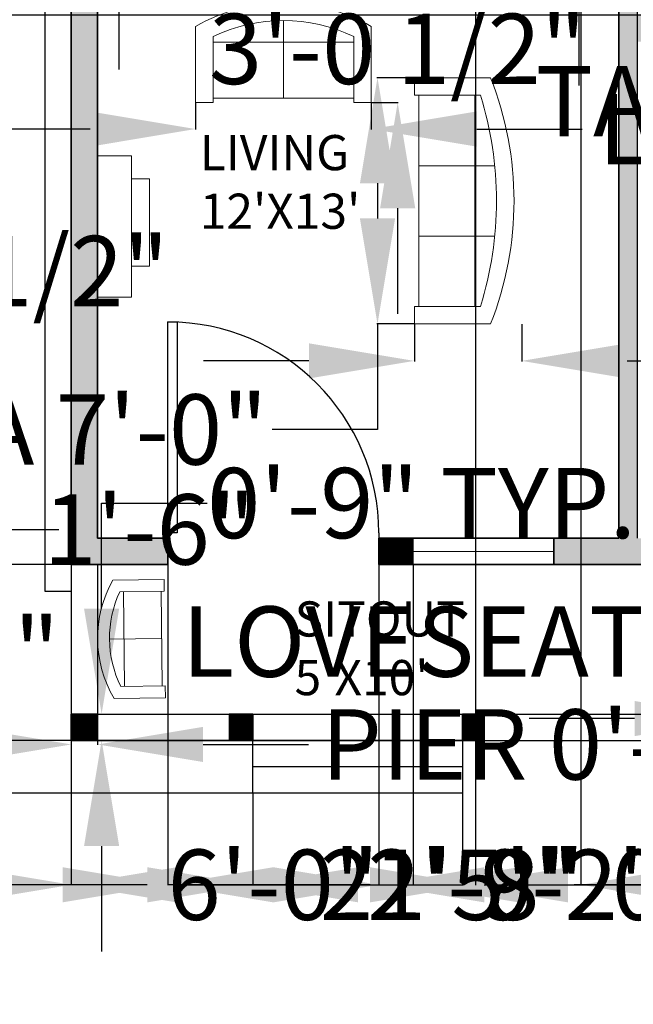
# Model space of a CAD drawing. Units: inches. Extents: x 2838 to 4029, y 1041 to 1915.
# Tile 2 of 16: x 3250 to 3460, y 1041 to 1377. Entities that reach past the tile are written whole.
import ezdxf

# ---------------------------------------------------------------- set-up
doc = ezdxf.new("R2010")
doc.units = ezdxf.units.IN
doc.header["$MEASUREMENT"] = 0
for name, color, linetype, lineweight in [('A-ANNO-DIMS', 2, 'Continuous', 18), ('A-AREA-IDEN', 7, 'Continuous', 18), ('A-COLS', 7, 'Continuous', 35), ('A-DOOR', 3, 'Continuous', 25), ('A-FLOR', 7, 'Continuous', 25), ('A-FLOR-STRS', 7, 'Continuous', 25), ('A-FURN', 8, 'Continuous', 18), ('A-GLAZ', 4, 'Continuous', 18), ('A-WALL', 7, 'Continuous', 35), ('A-WALL-PATT', 252, 'Continuous', 13)]:
    doc.layers.add(name, color=color, linetype=linetype, lineweight=lineweight)
doc.styles.get("Standard").update_dxf_attribs({"font": 'arial.ttf'})
doc.dimstyles.get("Standard").update_dxf_attribs({"dimtxt": 24, "dimasz": 36, "dimexe": 0.18, "dimexo": 0.0625, "dimgap": 0.09, "dimtad": 0, "dimtih": 1, "dimtoh": 1, "dimdec": 0, "dimzin": 0, "dimdsep": 46, "dimlunit": 3, "dimtxsty": 'Standard', "dimcen": 0.09, "dimadec": 0, "dimazin": 0, "dimtfac": 1, "dimtdec": 0, "dimtofl": 0, "dimtmove": 0, "dimatfit": 3, "dimfxl": 1, "dimtolj": 1, "dimtzin": 0, "dimarcsym": 0})

# ---------------------------------------------------------------- blocks, each defined once
blk = doc.blocks.new('*U4')
for p, q in [((0, 0), (0, -6)), ((40, 0), (40, -6))]:
    blk.add_line(p, q)
blk.add_lwpolyline([(0, 0), (0, 40), (1.75, 40), (1.75, 0)], close=True)
blk.add_arc((0, 0), 40, 0, 90)
blk = doc.blocks.new('Sofa - Roundback Loveseat 5 ft.')
for p, q in [((0, -32.44198), (0, -5.99998)), ((-24, -33.99998), (-24, -11.46958)), ((-23.9998, -13.38178), (23.99986, -13.38178)), ((24.00004, -33.99998), (24.00004, -11.46958)), ((-24, -32.44198), (24.00004, -32.44198))]:
    blk.add_line(p, q)
for points in [[(-24, -33.99998), (-30, -33.99998), (-30, -7.99998)], [(30.00004, -7.99998), (30.00004, -33.99998), (24.00004, -33.99998)]]:
    blk.add_lwpolyline(points)
for centre, radius, start, end in [((0, -60.24998), 60.24998, 60.13715, 119.8628), ((0, -61.38438), 55.38444, 64.32083, 115.6792)]:
    blk.add_arc(centre, radius, start, end)
blk = doc.blocks.new('Sofa - Roundback 7 ft.')
for p, q in [((-12.00002, -32.4421), (-12.00003, -6.5971)), ((11.99997, -32.4421), (11.99998, -6.5971)), ((-36.000027, -34), (-36.000027, -11.4696)), ((-35.999844, -13.3819), (35.9998, -13.3819)), ((35.99998, -34), (35.99998, -11.4696)), ((-36.000027, -32.4421), (35.99998, -32.4421))]:
    blk.add_line(p, q)
for points in [[(-36.000027, -34), (-42.000027, -34), (-42.000027, -8)], [(41.99998, -8), (41.99998, -34), (35.99998, -34)]]:
    blk.add_lwpolyline(points)
for centre, radius, start, end in [((0, -114.25), 114.25, 68.43141, 111.5686), ((-0.00001, -127.1968), 121.1968, 72.72033, 107.2797)]:
    blk.add_arc(centre, radius, start, end)
blk = doc.blocks.new('WIN-48')
blk.add_line((4.5, 48), (4.5, 0))
blk.add_lwpolyline([(0, 48), (9, 48), (9, 0), (0, 0)], close=True)
blk = doc.blocks.new('PORCH-PIER-9X9')
blk.add_lwpolyline([(9, 9), (0, 9), (0, 0), (9, 0)], close=True)
blk = doc.blocks.new('*D25')
at = {"layer": 'A-ANNO-DIMS', "color": 0, "lineweight": -2, "transparency": 16777216}
for p, q in [((3283.93, 1516.17), (3283.93, 1552.17)), ((3276.79, 1480.17), (3284.11, 1480.17)), ((3276.79, 1432.17), (3284.11, 1432.17)), ((3283.93, 1396.17), (3283.93, 1360.17))]:
    blk.add_line(p, q, dxfattribs=at)
at = {"layer": 'A-ANNO-DIMS', "color": 0, "transparency": 16777216}
for points in [[(3277.93, 1516.17), (3289.93, 1516.17), (3283.93, 1480.17)], [(3277.93, 1396.17), (3289.93, 1396.17), (3283.93, 1432.17)]]:
    blk.add_solid(points, dxfattribs=at)
at = {"layer": 'Defpoints', "color": 0, "transparency": 16777216}
for p in [(3276.73, 1480.17), (3283.93, 1480.17), (3276.73, 1432.17)]:
    blk.add_point(p, dxfattribs=at)
at = {"layer": 'A-ANNO-DIMS', "color": 0, "transparency": 16777216, "insert": (3283.93, 1456.17), "char_height": 24, "attachment_point": 5}
blk.add_mtext('\\A1;WINDOW 4\'-0" TYP.', dxfattribs=at)
blk = doc.blocks.new('*D29')
at = {"layer": 'A-ANNO-DIMS', "color": 0, "lineweight": -2, "transparency": 16777216}
for p, q in [((3310.15, 1348.85), (3310.15, 1339.73)), ((3370.15, 1348.85), (3370.15, 1339.73)), ((3274.15, 1339.91), (3238.15, 1339.91)), ((3406.15, 1339.91), (3442.15, 1339.91))]:
    blk.add_line(p, q, dxfattribs=at)
at = {"layer": 'A-ANNO-DIMS', "color": 0, "transparency": 16777216}
for points in [[(3274.15, 1345.91), (3274.15, 1333.91), (3310.15, 1339.91)], [(3406.15, 1345.91), (3406.15, 1333.91), (3370.15, 1339.91)]]:
    blk.add_solid(points, dxfattribs=at)
at = {"layer": 'Defpoints', "color": 0, "transparency": 16777216}
for p in [(3310.15, 1348.91), (3370.15, 1348.91), (3370.15, 1339.91)]:
    blk.add_point(p, dxfattribs=at)
at = {"layer": 'A-ANNO-DIMS', "color": 0, "transparency": 16777216, "insert": (3566.77, 1339.91), "char_height": 24, "attachment_point": 5}
blk.add_mtext('\\A1;LOVESEAT 5\'-0"', dxfattribs=at)
blk = doc.blocks.new('*D30')
at = {"layer": 'A-ANNO-DIMS', "color": 0, "lineweight": -2, "transparency": 16777216}
for p, q in [((3379.15, 1421.58), (3379.15, 1457.58)), ((3370.21, 1385.58), (3379.33, 1385.58)), ((3370.21, 1348.91), (3379.33, 1348.91)), ((3379.15, 1312.91), (3379.15, 1276.91))]:
    blk.add_line(p, q, dxfattribs=at)
at = {"layer": 'A-ANNO-DIMS', "color": 0, "transparency": 16777216}
for points in [[(3373.15, 1421.58), (3385.15, 1421.58), (3379.15, 1385.58)], [(3373.15, 1312.91), (3385.15, 1312.91), (3379.15, 1348.91)]]:
    blk.add_solid(points, dxfattribs=at)
at = {"layer": 'Defpoints', "color": 0, "transparency": 16777216}
for p in [(3370.15, 1385.58), (3379.15, 1385.58), (3370.15, 1348.91)]:
    blk.add_point(p, dxfattribs=at)
at = {"layer": 'A-ANNO-DIMS', "color": 0, "transparency": 16777216, "insert": (3379.15, 1367.25), "char_height": 24, "attachment_point": 5}
blk.add_mtext('\\A1;3\'-0 1/2"', dxfattribs=at)
blk = doc.blocks.new('*D31')
at = {"layer": 'A-ANNO-DIMS', "color": 0, "lineweight": -2, "transparency": 16777216}
for p, q in [((3489.98, 1221.23), (3489.98, 1257.23)), ((3495.97, 1185.23), (3489.8, 1185.23)), ((3495.97, 1144.84), (3489.8, 1144.84)), ((3489.98, 1108.84), (3489.98, 1072.84))]:
    blk.add_line(p, q, dxfattribs=at)
at = {"layer": 'A-ANNO-DIMS', "color": 0, "transparency": 16777216}
for points in [[(3483.98, 1221.23), (3495.98, 1221.23), (3489.98, 1185.23)], [(3483.98, 1108.84), (3495.98, 1108.84), (3489.98, 1144.84)]]:
    blk.add_solid(points, dxfattribs=at)
at = {"layer": 'Defpoints', "color": 0, "transparency": 16777216}
for p in [(3496.03, 1185.23), (3489.98, 1144.84), (3496.03, 1144.84)]:
    blk.add_point(p, dxfattribs=at)
at = {"layer": 'A-ANNO-DIMS', "color": 0, "transparency": 16777216, "insert": (3489.98, 1165.04), "char_height": 24, "attachment_point": 5}
blk.add_mtext('\\A1;LOVESEAT 3\'-4 1/2" TYP.', dxfattribs=at)
blk = doc.blocks.new('*D32')
at = {"layer": 'A-ANNO-DIMS', "color": 0, "lineweight": -2, "transparency": 16777216}
for p, q in [((3496.03, 1144.78), (3496.03, 1138.61)), ((3520.71, 1144.78), (3520.71, 1138.61)), ((3460.03, 1138.79), (3424.03, 1138.79)), ((3556.71, 1138.79), (3592.71, 1138.79))]:
    blk.add_line(p, q, dxfattribs=at)
at = {"layer": 'A-ANNO-DIMS', "color": 0, "transparency": 16777216}
for points in [[(3460.03, 1144.79), (3460.03, 1132.79), (3496.03, 1138.79)], [(3556.71, 1144.79), (3556.71, 1132.79), (3520.71, 1138.79)]]:
    blk.add_solid(points, dxfattribs=at)
at = {"layer": 'Defpoints', "color": 0, "transparency": 16777216}
for p in [(3496.03, 1144.84), (3520.71, 1144.84), (3520.71, 1138.79)]:
    blk.add_point(p, dxfattribs=at)
at = {"layer": 'A-ANNO-DIMS', "color": 0, "transparency": 16777216, "insert": (3694.12, 1138.79), "char_height": 24, "attachment_point": 5}
blk.add_mtext('\\A1;2\'-0 1/2" TYP.', dxfattribs=at)
blk = doc.blocks.new('*D33')
at = {"layer": 'A-ANNO-DIMS', "color": 0, "lineweight": -2, "transparency": 16777216}
for p, q in [((3601.73, 1469.45), (3601.73, 1505.45)), ((3603.48, 1433.45), (3601.55, 1433.45)), ((3603.48, 1421.37), (3601.55, 1421.37)), ((3601.73, 1385.37), (3601.73, 1349.37)), ((3601.73, 1349.37), (3565.73, 1349.37))]:
    blk.add_line(p, q, dxfattribs=at)
at = {"layer": 'A-ANNO-DIMS', "color": 0, "transparency": 16777216}
for points in [[(3595.73, 1469.45), (3607.73, 1469.45), (3601.73, 1433.45)], [(3595.73, 1385.37), (3607.73, 1385.37), (3601.73, 1421.37)]]:
    blk.add_solid(points, dxfattribs=at)
at = {"layer": 'Defpoints', "color": 0, "transparency": 16777216}
for p in [(3603.54, 1433.45), (3601.73, 1421.37), (3603.54, 1421.37)]:
    blk.add_point(p, dxfattribs=at)
at = {"layer": 'A-ANNO-DIMS', "color": 0, "transparency": 16777216, "insert": (3496.18, 1349.37), "char_height": 24, "attachment_point": 5}
blk.add_mtext('\\A1;TAP 1\'-0"', dxfattribs=at)
blk = doc.blocks.new('*D43')
at = {"layer": 'A-ANNO-DIMS', "color": 0, "lineweight": -2, "transparency": 16777216}
for p, q in [((3231.73, 1129.95), (3195.73, 1129.95)), ((3267.73, 1131.23), (3267.73, 1129.77)), ((3276.73, 1131.23), (3276.73, 1129.77)), ((3312.73, 1129.95), (3348.73, 1129.95))]:
    blk.add_line(p, q, dxfattribs=at)
at = {"layer": 'A-ANNO-DIMS', "color": 0, "transparency": 16777216}
for points in [[(3231.73, 1135.95), (3231.73, 1123.95), (3267.73, 1129.95)], [(3312.73, 1135.95), (3312.73, 1123.95), (3276.73, 1129.95)]]:
    blk.add_solid(points, dxfattribs=at)
at = {"layer": 'Defpoints', "color": 0, "transparency": 16777216}
for p in [(3267.73, 1131.3), (3276.73, 1131.3), (3276.73, 1129.95)]:
    blk.add_point(p, dxfattribs=at)
at = {"layer": 'A-ANNO-DIMS', "color": 0, "transparency": 16777216, "insert": (3465.15, 1129.95), "char_height": 24, "attachment_point": 5}
blk.add_mtext('\\A1;PIER 0\'-9" TYP.', dxfattribs=at)
blk = doc.blocks.new('*D44')
at = {"layer": 'A-ANNO-DIMS', "color": 0, "lineweight": -2, "transparency": 16777216}
for p, q in [((3278.08, 1176.3), (3278.08, 1212.3)), ((3278.08, 1212.3), (3314.08, 1212.3)), ((3276.79, 1140.3), (3278.26, 1140.3)), ((3276.79, 1131.3), (3278.26, 1131.3)), ((3278.08, 1095.3), (3278.08, 1059.3))]:
    blk.add_line(p, q, dxfattribs=at)
at = {"layer": 'A-ANNO-DIMS', "color": 0, "transparency": 16777216}
for points in [[(3272.08, 1176.3), (3284.08, 1176.3), (3278.08, 1140.3)], [(3272.08, 1095.3), (3284.08, 1095.3), (3278.08, 1131.3)]]:
    blk.add_solid(points, dxfattribs=at)
at = {"layer": 'Defpoints', "color": 0, "transparency": 16777216}
for p in [(3276.73, 1140.3), (3278.08, 1140.3), (3276.73, 1131.3)]:
    blk.add_point(p, dxfattribs=at)
at = {"layer": 'A-ANNO-DIMS', "color": 0, "transparency": 16777216, "insert": (3387.32, 1212.3), "char_height": 24, "attachment_point": 5}
blk.add_mtext('\\A1;0\'-9" TYP.', dxfattribs=at)
blk = doc.blocks.new('*D49')
at = {"layer": 'A-ANNO-DIMS', "color": 0, "lineweight": -2, "transparency": 16777216}
for p, q in [((3336.37, 1426.68), (3336.37, 1412.92)), ((3427.37, 1426.68), (3427.37, 1412.92)), ((3372.37, 1413.1), (3391.37, 1413.1)), ((3427.37, 1413.1), (3463.37, 1413.1))]:
    blk.add_line(p, q, dxfattribs=at)
at = {"layer": 'A-ANNO-DIMS', "color": 0, "transparency": 16777216}
for points in [[(3372.37, 1419.1), (3372.37, 1407.1), (3336.37, 1413.1)], [(3391.37, 1419.1), (3391.37, 1407.1), (3427.37, 1413.1)]]:
    blk.add_solid(points, dxfattribs=at)
at = {"layer": 'Defpoints', "color": 0, "transparency": 16777216}
for p in [(3336.37, 1426.75), (3427.37, 1426.75), (3427.37, 1413.1)]:
    blk.add_point(p, dxfattribs=at)
at = {"layer": 'A-ANNO-DIMS', "color": 0, "transparency": 16777216, "insert": (3595.36, 1413.1), "char_height": 24, "attachment_point": 5}
blk.add_mtext('\\A1;DINING SET 7\'-7"', dxfattribs=at)
blk = doc.blocks.new('*D50')
at = {"layer": 'A-ANNO-DIMS', "color": 0, "lineweight": -2, "transparency": 16777216}
for p, q in [((3441.02, 1517.75), (3441.02, 1553.75)), ((3427.44, 1481.75), (3441.2, 1481.75)), ((3427.44, 1426.75), (3441.2, 1426.75)), ((3441.02, 1390.75), (3441.02, 1354.75))]:
    blk.add_line(p, q, dxfattribs=at)
at = {"layer": 'A-ANNO-DIMS', "color": 0, "transparency": 16777216}
for points in [[(3435.02, 1517.75), (3447.02, 1517.75), (3441.02, 1481.75)], [(3435.02, 1390.75), (3447.02, 1390.75), (3441.02, 1426.75)]]:
    blk.add_solid(points, dxfattribs=at)
at = {"layer": 'Defpoints', "color": 0, "transparency": 16777216}
for p in [(3427.37, 1481.75), (3441.02, 1481.75), (3427.37, 1426.75)]:
    blk.add_point(p, dxfattribs=at)
at = {"layer": 'A-ANNO-DIMS', "color": 0, "transparency": 16777216, "insert": (3441.02, 1454.25), "char_height": 24, "attachment_point": 5}
blk.add_mtext('\\A1;4\'-7"', dxfattribs=at)
blk = doc.blocks.new('*D51')
at = {"layer": 'A-ANNO-DIMS', "color": 0, "lineweight": -2, "transparency": 16777216}
for p, q in [((3384.81, 1357.41), (3372.09, 1357.41)), ((3372.27, 1321.41), (3372.27, 1309.41)), ((3384.81, 1273.41), (3372.09, 1273.41)), ((3372.27, 1273.41), (3372.27, 1237.41)), ((3372.27, 1237.41), (3336.27, 1237.41))]:
    blk.add_line(p, q, dxfattribs=at)
at = {"layer": 'A-ANNO-DIMS', "color": 0, "transparency": 16777216}
for points in [[(3366.27, 1321.41), (3378.27, 1321.41), (3372.27, 1357.41)], [(3366.27, 1309.41), (3378.27, 1309.41), (3372.27, 1273.41)]]:
    blk.add_solid(points, dxfattribs=at)
at = {"layer": 'Defpoints', "color": 0, "transparency": 16777216}
for p in [(3384.87, 1357.41), (3372.27, 1273.41), (3384.87, 1273.41)]:
    blk.add_point(p, dxfattribs=at)
at = {"layer": 'A-ANNO-DIMS', "color": 0, "transparency": 16777216, "insert": (3254.04, 1237.41), "char_height": 24, "attachment_point": 5}
blk.add_mtext('\\A1;SOFA 7\'-0"', dxfattribs=at)
blk = doc.blocks.new('*D52')
at = {"layer": 'A-ANNO-DIMS', "color": 0, "lineweight": -2, "transparency": 16777216}
for p, q in [((3384.87, 1273.35), (3384.87, 1260.63)), ((3421.54, 1273.35), (3421.54, 1260.63)), ((3348.87, 1260.81), (3312.87, 1260.81)), ((3457.54, 1260.81), (3493.54, 1260.81))]:
    blk.add_line(p, q, dxfattribs=at)
at = {"layer": 'A-ANNO-DIMS', "color": 0, "transparency": 16777216}
for points in [[(3348.87, 1266.81), (3348.87, 1254.81), (3384.87, 1260.81)], [(3457.54, 1266.81), (3457.54, 1254.81), (3421.54, 1260.81)]]:
    blk.add_solid(points, dxfattribs=at)
at = {"layer": 'Defpoints', "color": 0, "transparency": 16777216}
for p in [(3384.87, 1273.41), (3421.54, 1273.41), (3421.54, 1260.81)]:
    blk.add_point(p, dxfattribs=at)
at = {"layer": 'A-ANNO-DIMS', "color": 0, "transparency": 16777216, "insert": (3553.48, 1260.81), "char_height": 24, "attachment_point": 5}
blk.add_mtext('\\A1;3\'-0 1/2"', dxfattribs=at)
blk = doc.blocks.new('*D57')
at = {"layer": 'A-ANNO-DIMS', "color": 0, "lineweight": -2, "transparency": 16777216}
for p, q in [((3585.57, 1472.38), (3585.57, 1508.38)), ((3590.9, 1436.38), (3585.39, 1436.38)), ((3590.9, 1400.38), (3585.39, 1400.38)), ((3585.57, 1364.38), (3585.57, 1328.38))]:
    blk.add_line(p, q, dxfattribs=at)
at = {"layer": 'A-ANNO-DIMS', "color": 0, "transparency": 16777216}
for points in [[(3579.57, 1472.38), (3591.57, 1472.38), (3585.57, 1436.38)], [(3579.57, 1364.38), (3591.57, 1364.38), (3585.57, 1400.38)]]:
    blk.add_solid(points, dxfattribs=at)
at = {"layer": 'Defpoints', "color": 0, "transparency": 16777216}
for p in [(3590.97, 1436.38), (3585.57, 1400.38), (3590.97, 1400.38)]:
    blk.add_point(p, dxfattribs=at)
at = {"layer": 'A-ANNO-DIMS', "color": 0, "transparency": 16777216, "insert": (3585.57, 1418.38), "char_height": 24, "attachment_point": 5}
blk.add_mtext('\\A1;DOUBLE SINK 3\'-0"', dxfattribs=at)
blk = doc.blocks.new('*D65')
at = {"layer": 'A-ANNO-DIMS', "color": 0, "lineweight": -2, "transparency": 16777216}
for p, q in [((3267.73, 1131.23), (3267.73, 1081.89)), ((3527.95, 1131.23), (3527.95, 1081.89)), ((3303.73, 1082.07), (3356.32, 1082.07)), ((3491.95, 1082.07), (3439.36, 1082.07))]:
    blk.add_line(p, q, dxfattribs=at)
at = {"layer": 'A-ANNO-DIMS', "color": 0, "transparency": 16777216}
for points in [[(3303.73, 1088.07), (3303.73, 1076.07), (3267.73, 1082.07)], [(3491.95, 1088.07), (3491.95, 1076.07), (3527.95, 1082.07)]]:
    blk.add_solid(points, dxfattribs=at)
at = {"layer": 'Defpoints', "color": 0, "transparency": 16777216}
for p in [(3267.73, 1131.3), (3527.95, 1131.3), (3527.95, 1082.07)]:
    blk.add_point(p, dxfattribs=at)
at = {"layer": 'A-ANNO-DIMS', "color": 0, "transparency": 16777216, "insert": (3397.84, 1082.07), "char_height": 24, "attachment_point": 5}
blk.add_mtext('\\A1;21\'-8"', dxfattribs=at)
blk = doc.blocks.new('*D66')
at = {"layer": 'A-ANNO-DIMS', "color": 0, "lineweight": -2, "transparency": 16777216}
for p, q in [((3227.506626, 1227.297346), (3227.506626, 1263.297346)), ((3267.669126, 1191.297346), (3227.326626, 1191.297346)), ((3267.669126, 1131.297346), (3227.326626, 1131.297346)), ((3227.506626, 1095.297346), (3227.506626, 1059.297346))]:
    blk.add_line(p, q, dxfattribs=at)
at = {"layer": 'A-ANNO-DIMS', "color": 0, "transparency": 16777216}
for points in [[(3221.506626, 1227.297346), (3233.506626, 1227.297346), (3227.506626, 1191.297346)], [(3221.506626, 1095.297346), (3233.506626, 1095.297346), (3227.506626, 1131.297346)]]:
    blk.add_solid(points, dxfattribs=at)
at = {"layer": 'Defpoints', "color": 0, "transparency": 16777216}
for p in [(3267.731626, 1191.297346), (3227.506626, 1131.297346), (3267.731626, 1131.297346)]:
    blk.add_point(p, dxfattribs=at)
at = {"layer": 'A-ANNO-DIMS', "color": 0, "transparency": 16777216, "insert": (3227.506626, 1161.297346), "char_height": 24, "attachment_point": 5}
blk.add_mtext('\\A1;5\'-0"', dxfattribs=at)
blk = doc.blocks.new('*D67')
at = {"layer": 'A-ANNO-DIMS', "color": 0, "lineweight": -2, "transparency": 16777216}
for p, q in [((3258.67, 1680.3), (3227.33, 1680.3)), ((3227.51, 1644.3), (3227.51, 1409.15)), ((3227.51, 1149.3), (3227.51, 1384.45)), ((3329.6, 1113.3), (3227.33, 1113.3))]:
    blk.add_line(p, q, dxfattribs=at)
at = {"layer": 'A-ANNO-DIMS', "color": 0, "transparency": 16777216}
for points in [[(3221.51, 1644.3), (3233.51, 1644.3), (3227.51, 1680.3)], [(3221.51, 1149.3), (3233.51, 1149.3), (3227.51, 1113.3)]]:
    blk.add_solid(points, dxfattribs=at)
at = {"layer": 'Defpoints', "color": 0, "transparency": 16777216}
for p in [(3227.51, 1680.3), (3258.73, 1680.3), (3329.66, 1113.3)]:
    blk.add_point(p, dxfattribs=at)
at = {"layer": 'A-ANNO-DIMS', "color": 0, "transparency": 16777216, "insert": (3227.51, 1396.8), "char_height": 24, "attachment_point": 5}
blk.add_mtext('\\A1;47\'-3"', dxfattribs=at)
blk = doc.blocks.new('*D69')
at = {"layer": 'A-ANNO-DIMS', "color": 0, "lineweight": -2, "transparency": 16777216}
for p, q in [((3300.731626, 1191.234846), (3300.731626, 1081.892346)), ((3372.731626, 1191.234846), (3372.731626, 1081.892346)), ((3264.731626, 1082.072346), (3228.731626, 1082.072346)), ((3408.731626, 1082.072346), (3444.731626, 1082.072346))]:
    blk.add_line(p, q, dxfattribs=at)
at = {"layer": 'A-ANNO-DIMS', "color": 0, "transparency": 16777216}
for points in [[(3264.731626, 1088.072346), (3264.731626, 1076.072346), (3300.731626, 1082.072346)], [(3408.731626, 1088.072346), (3408.731626, 1076.072346), (3372.731626, 1082.072346)]]:
    blk.add_solid(points, dxfattribs=at)
at = {"layer": 'Defpoints', "color": 0, "transparency": 16777216}
for p in [(3300.731626, 1191.297346), (3372.731626, 1191.297346), (3372.731626, 1082.072346)]:
    blk.add_point(p, dxfattribs=at)
at = {"layer": 'A-ANNO-DIMS', "color": 0, "transparency": 16777216, "insert": (3336.731626, 1082.072346), "char_height": 24, "attachment_point": 5}
blk.add_mtext('\\A1;6\'-0"', dxfattribs=at)
blk = doc.blocks.new('*D70')
at = {"layer": 'A-ANNO-DIMS', "color": 0, "lineweight": -2, "transparency": 16777216}
for p, q in [((3329.66, 1113.23), (3329.66, 1081.89)), ((3401.28, 1113.23), (3401.28, 1081.89)), ((3293.66, 1082.07), (3257.66, 1082.07)), ((3437.28, 1082.07), (3473.28, 1082.07))]:
    blk.add_line(p, q, dxfattribs=at)
at = {"layer": 'A-ANNO-DIMS', "color": 0, "transparency": 16777216}
for points in [[(3293.66, 1088.07), (3293.66, 1076.07), (3329.66, 1082.07)], [(3437.28, 1088.07), (3437.28, 1076.07), (3401.28, 1082.07)]]:
    blk.add_solid(points, dxfattribs=at)
at = {"layer": 'Defpoints', "color": 0, "transparency": 16777216}
for p in [(3329.66, 1113.3), (3401.28, 1113.3), (3401.28, 1082.07)]:
    blk.add_point(p, dxfattribs=at)
at = {"layer": 'A-ANNO-DIMS', "color": 0, "transparency": 16777216, "insert": (3542.56, 1082.07), "char_height": 24, "attachment_point": 5}
blk.add_mtext('\\A1;5\'-11 1/2"', dxfattribs=at)
blk = doc.blocks.new('*D71')
at = {"layer": 'A-ANNO-DIMS', "color": 0, "lineweight": -2, "transparency": 16777216}
for p, q in [((3267.73, 1131.23), (3267.73, 1081.89)), ((3329.66, 1113.23), (3329.66, 1081.89)), ((3231.73, 1082.07), (3195.73, 1082.07)), ((3365.66, 1082.07), (3401.66, 1082.07))]:
    blk.add_line(p, q, dxfattribs=at)
at = {"layer": 'A-ANNO-DIMS', "color": 0, "transparency": 16777216}
for points in [[(3231.73, 1088.07), (3231.73, 1076.07), (3267.73, 1082.07)], [(3365.66, 1088.07), (3365.66, 1076.07), (3329.66, 1082.07)]]:
    blk.add_solid(points, dxfattribs=at)
at = {"layer": 'Defpoints', "color": 0, "transparency": 16777216}
for p in [(3267.73, 1131.3), (3329.66, 1113.3), (3329.66, 1082.07)]:
    blk.add_point(p, dxfattribs=at)
at = {"layer": 'A-ANNO-DIMS', "color": 0, "transparency": 16777216, "insert": (3433.65, 1082.07), "char_height": 24, "attachment_point": 5}
blk.add_mtext('\\A1;5\'-2"', dxfattribs=at)
blk = doc.blocks.new('*D72')
at = {"layer": 'A-ANNO-DIMS', "color": 0, "lineweight": -2, "transparency": 16777216}
for p, q in [((3227.51, 1167.3), (3227.51, 1203.3)), ((3227.51, 1203.3), (3263.51, 1203.3)), ((3329.6, 1131.3), (3227.33, 1131.3)), ((3329.6, 1113.3), (3227.33, 1113.3)), ((3227.51, 1077.3), (3227.51, 1041.3))]:
    blk.add_line(p, q, dxfattribs=at)
at = {"layer": 'A-ANNO-DIMS', "color": 0, "transparency": 16777216}
for points in [[(3221.51, 1167.3), (3233.51, 1167.3), (3227.51, 1131.3)], [(3221.51, 1077.3), (3233.51, 1077.3), (3227.51, 1113.3)]]:
    blk.add_solid(points, dxfattribs=at)
at = {"layer": 'Defpoints', "color": 0, "transparency": 16777216}
for p in [(3227.51, 1131.3), (3329.66, 1131.3), (3329.66, 1113.3)]:
    blk.add_point(p, dxfattribs=at)
at = {"layer": 'A-ANNO-DIMS', "color": 0, "transparency": 16777216, "insert": (3294.37, 1203.3), "char_height": 24, "attachment_point": 5}
blk.add_mtext('\\A1;1\'-6"', dxfattribs=at)
blk = doc.blocks.new('*D73')
at = {"layer": 'A-ANNO-DIMS', "color": 0, "lineweight": -2, "transparency": 16777216}
for p, q in [((3425.038746, 1711.522346), (3389.038746, 1711.522346)), ((3461.038746, 1200.359846), (3461.038746, 1711.702346)), ((3618.731626, 1200.359846), (3618.731626, 1711.702346)), ((3654.731626, 1711.522346), (3690.731626, 1711.522346))]:
    blk.add_line(p, q, dxfattribs=at)
at = {"layer": 'A-ANNO-DIMS', "color": 0, "transparency": 16777216}
for points in [[(3425.038746, 1717.522346), (3425.038746, 1705.522346), (3461.038746, 1711.522346)], [(3654.731626, 1717.522346), (3654.731626, 1705.522346), (3618.731626, 1711.522346)]]:
    blk.add_solid(points, dxfattribs=at)
at = {"layer": 'Defpoints', "color": 0, "transparency": 16777216}
for p in [(3618.731626, 1711.522346), (3461.038746, 1200.297346), (3618.731626, 1200.297346)]:
    blk.add_point(p, dxfattribs=at)
at = {"layer": 'A-ANNO-DIMS', "color": 0, "transparency": 16777216, "insert": (3539.885186, 1711.522346), "char_height": 24, "attachment_point": 5}
blk.add_mtext('\\A1;13\'-1 1/2"', dxfattribs=at)
blk = doc.blocks.new('*D74')
at = {"layer": 'A-ANNO-DIMS', "color": 0, "lineweight": -2, "transparency": 16777216}
for p, q in [((3513.73, 1297.66), (3513.73, 1081.89)), ((3525.73, 1297.66), (3525.73, 1081.89)), ((3477.73, 1082.07), (3441.73, 1082.07)), ((3561.73, 1082.07), (3597.73, 1082.07))]:
    blk.add_line(p, q, dxfattribs=at)
at = {"layer": 'A-ANNO-DIMS', "color": 0, "transparency": 16777216}
for points in [[(3477.73, 1088.07), (3477.73, 1076.07), (3513.73, 1082.07)], [(3561.73, 1088.07), (3561.73, 1076.07), (3525.73, 1082.07)]]:
    blk.add_solid(points, dxfattribs=at)
at = {"layer": 'Defpoints', "color": 0, "transparency": 16777216}
for p in [(3513.73, 1297.73), (3525.73, 1297.73), (3525.73, 1082.07)]:
    blk.add_point(p, dxfattribs=at)
at = {"layer": 'A-ANNO-DIMS', "color": 0, "transparency": 16777216, "insert": (3628.59, 1082.07), "char_height": 24, "attachment_point": 5}
blk.add_mtext('\\A1;1\'-0"', dxfattribs=at)
blk = doc.blocks.new('*D76')
at = {"layer": 'A-ANNO-DIMS', "color": 0, "lineweight": -2, "transparency": 16777216}
for p, q in [((3276.67, 1391.57), (3227.33, 1391.57)), ((3227.51, 1355.57), (3227.51, 1303.94)), ((3227.51, 1227.3), (3227.51, 1278.94)), ((3267.67, 1191.3), (3227.33, 1191.3))]:
    blk.add_line(p, q, dxfattribs=at)
at = {"layer": 'A-ANNO-DIMS', "color": 0, "transparency": 16777216}
for points in [[(3221.51, 1355.57), (3233.51, 1355.57), (3227.51, 1391.57)], [(3221.51, 1227.3), (3233.51, 1227.3), (3227.51, 1191.3)]]:
    blk.add_solid(points, dxfattribs=at)
at = {"layer": 'Defpoints', "color": 0, "transparency": 16777216}
for p in [(3227.51, 1391.57), (3276.73, 1391.57), (3267.73, 1191.3)]:
    blk.add_point(p, dxfattribs=at)
at = {"layer": 'A-ANNO-DIMS', "color": 0, "transparency": 16777216, "insert": (3227.51, 1291.44), "char_height": 24, "attachment_point": 5}
blk.add_mtext('\\A1;16\'-8 1/2"', dxfattribs=at)
blk = doc.blocks.new('*D81')
at = {"layer": 'A-ANNO-DIMS', "color": 0, "lineweight": -2, "transparency": 16777216}
for p, q in [((3267.73, 1191.23), (3267.73, 1081.89)), ((3300.73, 1191.23), (3300.73, 1081.89)), ((3231.73, 1082.07), (3195.73, 1082.07)), ((3336.73, 1082.07), (3372.73, 1082.07))]:
    blk.add_line(p, q, dxfattribs=at)
at = {"layer": 'A-ANNO-DIMS', "color": 0, "transparency": 16777216}
for points in [[(3231.73, 1088.07), (3231.73, 1076.07), (3267.73, 1082.07)], [(3336.73, 1088.07), (3336.73, 1076.07), (3300.73, 1082.07)]]:
    blk.add_solid(points, dxfattribs=at)
at = {"layer": 'Defpoints', "color": 0, "transparency": 16777216}
for p in [(3267.73, 1191.3), (3300.73, 1191.3), (3300.73, 1082.07)]:
    blk.add_point(p, dxfattribs=at)
at = {"layer": 'A-ANNO-DIMS', "color": 0, "transparency": 16777216, "insert": (3404.93, 1082.07), "char_height": 24, "attachment_point": 5}
blk.add_mtext('\\A1;2\'-9"', dxfattribs=at)
blk = doc.blocks.new('*D82')
at = {"layer": 'A-ANNO-DIMS', "color": 0, "lineweight": -2, "transparency": 16777216}
for p, q in [((3405.73, 1573.06), (3405.73, 1081.89)), ((3441.73, 1569.23), (3441.73, 1081.89)), ((3369.73, 1082.07), (3333.73, 1082.07)), ((3477.73, 1082.07), (3513.73, 1082.07))]:
    blk.add_line(p, q, dxfattribs=at)
at = {"layer": 'A-ANNO-DIMS', "color": 0, "transparency": 16777216}
for points in [[(3369.73, 1088.07), (3369.73, 1076.07), (3405.73, 1082.07)], [(3477.73, 1088.07), (3477.73, 1076.07), (3441.73, 1082.07)]]:
    blk.add_solid(points, dxfattribs=at)
at = {"layer": 'Defpoints', "color": 0, "transparency": 16777216}
for p in [(3405.73, 1573.12), (3441.73, 1569.3), (3441.73, 1082.07)]:
    blk.add_point(p, dxfattribs=at)
at = {"layer": 'A-ANNO-DIMS', "color": 0, "transparency": 16777216, "insert": (3545.71, 1082.07), "char_height": 24, "attachment_point": 5}
blk.add_mtext('\\A1;3\'-0"', dxfattribs=at)
blk = doc.blocks.new('*D87')
at = {"layer": 'A-ANNO-DIMS', "color": 0, "lineweight": -2, "transparency": 16777216}
for p, q in [((3227.506626, 1497.394218), (3227.506626, 1533.394218)), ((3513.669126, 1461.394218), (3227.326626, 1461.394218)), ((3513.669126, 1425.394218), (3227.326626, 1425.394218)), ((3227.506626, 1389.394218), (3227.506626, 1353.394218))]:
    blk.add_line(p, q, dxfattribs=at)
at = {"layer": 'A-ANNO-DIMS', "color": 0, "transparency": 16777216}
for points in [[(3221.506626, 1497.394218), (3233.506626, 1497.394218), (3227.506626, 1461.394218)], [(3221.506626, 1389.394218), (3233.506626, 1389.394218), (3227.506626, 1425.394218)]]:
    blk.add_solid(points, dxfattribs=at)
at = {"layer": 'Defpoints', "color": 0, "transparency": 16777216}
for p in [(3227.506626, 1461.394218), (3513.731626, 1461.394218), (3513.731626, 1425.394218)]:
    blk.add_point(p, dxfattribs=at)
at = {"layer": 'A-ANNO-DIMS', "color": 0, "transparency": 16777216, "insert": (3227.506626, 1443.394218), "char_height": 24, "attachment_point": 5}
blk.add_mtext('\\A1;3\'-0"', dxfattribs=at)
blk = doc.blocks.new('*D93')
at = {"layer": 'A-ANNO-DIMS', "color": 0, "lineweight": -2, "transparency": 16777216}
for p, q in [((3227.51, 1438.06), (3227.51, 1474.06)), ((3227.51, 1474.06), (3263.51, 1474.06)), ((3522.67, 1402.06), (3227.33, 1402.06)), ((3522.67, 1378.73), (3227.33, 1378.73)), ((3227.51, 1342.73), (3227.51, 1306.73))]:
    blk.add_line(p, q, dxfattribs=at)
at = {"layer": 'A-ANNO-DIMS', "color": 0, "transparency": 16777216}
for points in [[(3221.51, 1438.06), (3233.51, 1438.06), (3227.51, 1402.06)], [(3221.51, 1342.73), (3233.51, 1342.73), (3227.51, 1378.73)]]:
    blk.add_solid(points, dxfattribs=at)
at = {"layer": 'Defpoints', "color": 0, "transparency": 16777216}
for p in [(3227.51, 1402.06), (3522.73, 1402.06), (3522.73, 1378.73)]:
    blk.add_point(p, dxfattribs=at)
at = {"layer": 'A-ANNO-DIMS', "color": 0, "transparency": 16777216, "insert": (3331.65, 1474.06), "char_height": 24, "attachment_point": 5}
blk.add_mtext('\\A1;1\'-11 1/2"', dxfattribs=at)
blk = doc.blocks.new('*D95')
at = {"layer": 'A-ANNO-DIMS', "color": 0, "lineweight": -2, "transparency": 16777216}
for p, q in [((3227.51, 1468.17), (3227.51, 1504.17)), ((3276.67, 1432.17), (3227.33, 1432.17)), ((3276.67, 1400.57), (3227.33, 1400.57)), ((3227.51, 1364.57), (3227.51, 1328.57))]:
    blk.add_line(p, q, dxfattribs=at)
at = {"layer": 'A-ANNO-DIMS', "color": 0, "transparency": 16777216}
for points in [[(3221.51, 1468.17), (3233.51, 1468.17), (3227.51, 1432.17)], [(3221.51, 1364.57), (3233.51, 1364.57), (3227.51, 1400.57)]]:
    blk.add_solid(points, dxfattribs=at)
at = {"layer": 'Defpoints', "color": 0, "transparency": 16777216}
for p in [(3227.51, 1432.17), (3276.73, 1432.17), (3276.73, 1400.57)]:
    blk.add_point(p, dxfattribs=at)
at = {"layer": 'A-ANNO-DIMS', "color": 0, "transparency": 16777216, "insert": (3227.51, 1416.37), "char_height": 24, "attachment_point": 5}
blk.add_mtext('\\A1;2\'-7 1/2"', dxfattribs=at)
blk = doc.blocks.new('*D100')
at = {"layer": 'A-ANNO-DIMS', "color": 0, "lineweight": -2, "transparency": 16777216}
for p, q in [((3372.73, 1191.23), (3372.73, 1081.89)), ((3384.45, 1191.23), (3384.45, 1081.89)), ((3336.73, 1082.07), (3300.73, 1082.07)), ((3420.45, 1082.07), (3456.45, 1082.07))]:
    blk.add_line(p, q, dxfattribs=at)
at = {"layer": 'A-ANNO-DIMS', "color": 0, "transparency": 16777216}
for points in [[(3336.73, 1088.07), (3336.73, 1076.07), (3372.73, 1082.07)], [(3420.45, 1088.07), (3420.45, 1076.07), (3384.45, 1082.07)]]:
    blk.add_solid(points, dxfattribs=at)
at = {"layer": 'Defpoints', "color": 0, "transparency": 16777216}
for p in [(3372.73, 1191.3), (3384.45, 1191.3), (3384.45, 1082.07)]:
    blk.add_point(p, dxfattribs=at)
at = {"layer": 'A-ANNO-DIMS', "color": 0, "transparency": 16777216, "insert": (3525.73, 1082.07), "char_height": 24, "attachment_point": 5}
blk.add_mtext('\\A1;0\'-11 1/2"', dxfattribs=at)
blk = doc.blocks.new('*D101')
at = {"layer": 'A-ANNO-DIMS', "color": 0, "lineweight": -2, "transparency": 16777216}
for p, q in [((3425.04, 1711.52), (3389.04, 1711.52)), ((3461.04, 1200.36), (3461.04, 1711.7)), ((3486.18, 1200.36), (3486.18, 1711.7)), ((3522.18, 1711.52), (3558.18, 1711.52))]:
    blk.add_line(p, q, dxfattribs=at)
at = {"layer": 'A-ANNO-DIMS', "color": 0, "transparency": 16777216}
for points in [[(3425.04, 1717.52), (3425.04, 1705.52), (3461.04, 1711.52)], [(3522.18, 1717.52), (3522.18, 1705.52), (3486.18, 1711.52)]]:
    blk.add_solid(points, dxfattribs=at)
at = {"layer": 'Defpoints', "color": 0, "transparency": 16777216}
for p in [(3486.18, 1711.52), (3461.04, 1200.3), (3486.18, 1200.3)]:
    blk.add_point(p, dxfattribs=at)
at = {"layer": 'A-ANNO-DIMS', "color": 0, "transparency": 16777216, "insert": (3590.37, 1711.52), "char_height": 24, "attachment_point": 5}
blk.add_mtext('\\A1;2\'-1"', dxfattribs=at)

msp = doc.modelspace()

# ---------------------------------------------------------------- hatches: boundary and pattern name
at = {"layer": 'A-WALL-PATT'}
h = msp.add_hatch(color=256, dxfattribs=at)
h.dxf.hatch_style = 1
h.paths.add_polyline_path([(3427.52, 1671.3), (3360.91, 1671.3), (3360.91, 1662.3), (3396.73, 1662.3), (3396.73, 1554.39), (3397.12, 1554.39, -0.007312), (3398.53, 1554.41), (3405.73, 1554.41), (3405.73, 1662.3), (3427.52, 1662.3)])
h.paths.add_polyline_path([(3546.42, 1671.3), (3451.52, 1671.3), (3451.52, 1662.3), (3489.73, 1662.3), (3489.73, 1592.86, -0.016107), (3489.73, 1591.9), (3489.73, 1578.3), (3441.73, 1578.3), (3441.73, 1569.3), (3489.73, 1569.3), (3489.73, 1554.41), (3498.73, 1554.41), (3498.73, 1662.3), (3546.42, 1662.3)])
h.paths.add_polyline_path([(3627.73, 1671.3), (3594.42, 1671.3), (3594.42, 1662.3), (3618.73, 1662.3), (3618.73, 1634.03), (3627.73, 1634.03)])
h.paths.add_polyline_path([(3627.73, 1586.03), (3618.73, 1586.03), (3618.73, 1506.39), (3545.12, 1506.39), (3489.73, 1506.39), (3489.73, 1497.39), (3513.73, 1497.39), (3618.73, 1497.39), (3618.73, 1469.85), (3627.73, 1469.85)])
h.paths.add_polyline_path([(3627.73, 1421.85), (3618.73, 1421.85), (3618.73, 1378.73), (3522.73, 1378.73), (3513.73, 1378.73), (3461.04, 1378.73), (3461.04, 1369.73), (3513.73, 1369.73), (3618.73, 1369.73), (3618.73, 1320.94), (3627.73, 1320.94)])
h.paths.add_polyline_path([(3627.73, 1272.94), (3618.73, 1272.94), (3618.73, 1200.3), (3599.07, 1200.3), (3599.07, 1191.3), (3627.73, 1191.3)])
h.paths.add_polyline_path([(3551.07, 1200.3), (3510.18, 1200.3), (3510.18, 1191.3), (3551.07, 1191.3)])
h.paths.add_polyline_path([(3486.18, 1200.3), (3461.04, 1200.3), (3461.04, 1398.25), (3454.63, 1398.25), (3454.63, 1200.3), (3432.45, 1200.3), (3432.45, 1191.3), (3486.18, 1191.3)])
h.paths.add_polyline_path([(3300.73, 1200.3), (3276.73, 1200.3), (3276.73, 1391.57), (3331.05, 1391.57), (3331.05, 1400.57), (3276.73, 1400.57), (3276.73, 1432.17), (3267.73, 1432.17), (3267.73, 1191.3), (3300.73, 1191.3)])
h = msp.add_hatch(dxfattribs=at)
h.set_pattern_fill('ANSI31', color=256)
h.paths.add_polyline_path([(3384.45, 1200.3), (3372.73, 1200.3), (3372.73, 1191.3), (3384.45, 1191.3)])
h.paths.add_polyline_path([(3276.73, 1140.3), (3267.73, 1140.3), (3267.73, 1131.3), (3276.73, 1131.3)])
h.paths.add_polyline_path([(3329.66, 1140.3), (3321.69, 1140.3), (3321.69, 1131.3), (3329.66, 1131.3)])
h.paths.add_polyline_path([(3408.74, 1140.3), (3401.28, 1140.3), (3401.28, 1131.3), (3408.74, 1131.3)])

# ---------------------------------------------------------------- linework, layer by layer
at = {"layer": 'A-COLS'}
for points in [[(3329.66, 1140.3), (3321.69, 1140.3), (3321.69, 1131.3), (3329.66, 1131.3)], [(3401.28, 1140.3), (3408.74, 1140.3), (3408.74, 1131.3), (3401.28, 1131.3)]]:
    msp.add_lwpolyline(points, close=True, dxfattribs=at)
at = {"layer": 'A-FLOR'}
for p, q in [((3267.73, 1191.3), (3267.73, 1131.3)), ((3276.73, 1191.3), (3276.73, 1140.3)), ((3276.73, 1140.3), (3498.72, 1140.3)), ((3267.73, 1131.3), (3507.72, 1131.3))]:
    msp.add_line(p, q, dxfattribs=at)
msp.add_lwpolyline([(3527.95, 1182.3), (3636.73, 1182.3), (3636.73, 1680.3), (3258.73, 1680.3), (3258.73, 1182.3), (3267.73, 1182.3)], dxfattribs=at)
at = {"layer": 'A-FLOR-STRS'}
for p, q in [((3329.66, 1140.3), (3401.28, 1140.3)), ((3329.66, 1131.3), (3329.66, 1140.3)), ((3401.28, 1140.3), (3401.28, 1131.3)), ((3401.28, 1131.3), (3329.66, 1131.3)), ((3329.66, 1113.3), (3329.66, 1131.3)), ((3401.28, 1131.3), (3401.28, 1113.3)), ((3401.28, 1122.3), (3329.66, 1122.3)), ((3401.28, 1113.3), (3329.66, 1113.3)), ((3401.28, 1113.3), (3329.66, 1113.3))]:
    msp.add_line(p, q, dxfattribs=at)
at = {"layer": 'A-FURN'}
for points in [[(3276.73, 1330.8), (3288.28, 1330.8), (3288.28, 1282.51), (3276.73, 1282.51)], [(3288.28, 1322.94), (3294.42, 1322.94), (3294.42, 1293.09), (3288.28, 1293.09)]]:
    msp.add_lwpolyline(points, close=True, dxfattribs=at)
at = {"layer": 'A-WALL'}
for p, q in [((3267.73, 1671.3), (3267.73, 1191.3)), ((3454.63, 1200.3), (3454.63, 1398.25)), ((3454.63, 1398.25), (3454.63, 1200.3)), ((3276.73, 1391.57), (3276.73, 1200.3)), ((3276.73, 1200.3), (3276.73, 1391.57)), ((3276.73, 1200.3), (3300.73, 1200.3)), ((3300.73, 1200.3), (3276.73, 1200.3)), ((3300.73, 1200.3), (3300.73, 1191.3)), ((3300.73, 1191.3), (3300.73, 1200.3)), ((3372.73, 1200.3), (3372.73, 1191.3)), ((3372.73, 1200.3), (3454.63, 1200.3)), ((3454.63, 1200.3), (3432.45, 1200.3)), ((3432.45, 1200.3), (3432.45, 1191.3)), ((3267.73, 1191.3), (3300.73, 1191.3)), ((3432.45, 1191.3), (3486.18, 1191.3))]:
    msp.add_line(p, q, dxfattribs=at)
msp.add_lwpolyline([(3372.73, 1191.3), (3627.73, 1191.3), (3627.73, 1671.3), (3267.73, 1671.3), (3267.73, 1191.3), (3300.73, 1191.3)], dxfattribs=at)

# ---------------------------------------------------------------- block references
at = {"layer": 'A-COLS'}
msp.add_blockref('PORCH-PIER-9X9', (3267.73, 1131.3), dxfattribs=at)
at = {"layer": 'A-DOOR', "xscale": 1.800064356479457, "yscale": 1.800064356479457, "zscale": 1.800064356479457}
msp.add_blockref('*U4', (3300.73, 1202.1), dxfattribs=at)
at = {"layer": 'A-FURN'}
msp.add_blockref('Sofa - Roundback Loveseat 5 ft.', (3340.15, 1382.91), dxfattribs=at)
at = {"layer": 'A-FURN', "rotation": 270}
msp.add_blockref('Sofa - Roundback 7 ft.', (3418.87, 1315.41), dxfattribs=at)
at = {"layer": 'A-FURN', "xscale": -0.6730714582278688, "yscale": 0.6730714582278688, "zscale": 0.6730714582278688, "rotation": 90.65283437104478}
msp.add_blockref('Sofa - Roundback Loveseat 5 ft.', (3276.73, 1165.8), dxfattribs=at)
at = {"layer": 'A-GLAZ', "rotation": 269.9999999999991}
msp.add_blockref('WIN-48', (3384.45, 1200.3), dxfattribs=at)

# ---------------------------------------------------------------- texts
at = {"layer": 'A-AREA-IDEN', "char_height": 12, "attachment_point": 1}
for s, insert in [("LIVING \\P12'X13'", (3311.59, 1337.87)), ("SITOUT\\P5'X10'", (3343.96, 1178.76))]:
    msp.add_mtext_dynamic_manual_height_columns(s, width=64.6015, gutter_width=1, heights=[0], dxfattribs=dict(at, insert=insert))

# ---------------------------------------------------------------- dimensions: what is measured, and where the dimension line sits
at = {"layer": 'A-ANNO-DIMS'}
for base, p1, p2, picture, middle in [((3618.73, 1711.52), (3461.04, 1200.3), (3618.73, 1200.3), '*D73', (3539.89, 1711.52)), ((3486.18, 1711.52), (3461.04, 1200.3), (3486.18, 1200.3), '*D101', (3590.37, 1711.52)), ((3441.73, 1082.07), (3405.73, 1573.12), (3441.73, 1569.3), '*D82', (3545.71, 1082.07)), ((3525.73, 1082.07), (3513.73, 1297.73), (3525.73, 1297.73), '*D74', (3628.59, 1082.07)), ((3421.54, 1260.81), (3384.87, 1273.41), (3421.54, 1273.41), '*D52', (3553.48, 1260.81)), ((3300.73, 1082.07), (3267.73, 1191.3), (3300.73, 1191.3), '*D81', (3404.93, 1082.07)), ((3372.73, 1082.07), (3300.73, 1191.3), (3372.73, 1191.3), '*D69', (3336.73, 1082.07)), ((3384.45, 1082.07), (3372.73, 1191.3), (3384.45, 1191.3), '*D100', (3525.73, 1082.07)), ((3329.66, 1082.07), (3267.73, 1131.3), (3329.66, 1113.3), '*D71', (3433.65, 1082.07)), ((3527.95, 1082.07), (3267.73, 1131.3), (3527.95, 1131.3), '*D65', (3397.84, 1082.07)), ((3401.28, 1082.07), (3329.66, 1113.3), (3401.28, 1113.3), '*D70', (3542.56, 1082.07))]:
    dim = msp.add_linear_dim(base=base, p1=p1, p2=p2, dimstyle='Standard', override={"dimdec": 1, "dimlfac": 1, "dimrnd": 0, "dimzin": 1, "dimdsep": 46, "dimlunit": 4, "dimfrac": 2}, dxfattribs=at)
    dim.commit()
    dim.dimension.update_dxf_attribs({"geometry": picture, "text_midpoint": middle})
for base, p1, p2, picture, middle in [((3227.51, 1680.3), (3329.66, 1113.3), (3258.73, 1680.3), '*D67', (3227.51, 1396.8)), ((3441.02, 1481.75), (3427.37, 1426.75), (3427.37, 1481.75), '*D50', (3441.02, 1454.25)), ((3227.51, 1461.39), (3513.73, 1425.39), (3513.73, 1461.39), '*D87', (3227.51, 1443.39)), ((3227.51, 1402.06), (3522.73, 1378.73), (3522.73, 1402.06), '*D93', (3331.65, 1474.06)), ((3227.51, 1432.17), (3276.73, 1400.57), (3276.73, 1432.17), '*D95', (3227.51, 1416.37)), ((3379.15, 1385.58), (3370.15, 1348.91), (3370.15, 1385.58), '*D30', (3379.15, 1367.25)), ((3227.51, 1391.57), (3267.73, 1191.3), (3276.73, 1391.57), '*D76', (3227.51, 1291.44)), ((3227.51, 1131.3), (3267.73, 1191.3), (3267.73, 1131.3), '*D66', (3227.51, 1161.3)), ((3227.51, 1131.3), (3329.66, 1113.3), (3329.66, 1131.3), '*D72', (3294.37, 1203.3))]:
    dim = msp.add_linear_dim(base=base, p1=p1, p2=p2, angle=90, dimstyle='Standard', override={"dimdec": 1, "dimlfac": 1, "dimrnd": 0, "dimzin": 1, "dimdsep": 46, "dimlunit": 4, "dimfrac": 2}, dxfattribs=at)
    dim.commit()
    dim.dimension.update_dxf_attribs({"geometry": picture, "text_midpoint": middle})
for base, p1, p2, angle, text, picture, middle in [((3283.93, 1480.17), (3276.73, 1432.17), (3276.73, 1480.17), 90, 'WINDOW <> TYP.', '*D25', (3283.93, 1456.17)), ((3585.57, 1400.38), (3590.97, 1436.38), (3590.97, 1400.38), 270, 'DOUBLE SINK <>', '*D57', (3585.57, 1418.38)), ((3601.73, 1421.37), (3603.54, 1433.45), (3603.54, 1421.37), 270, 'TAP <>', '*D33', (3496.18, 1349.37)), ((3372.27, 1273.41), (3384.87, 1357.41), (3384.87, 1273.41), 270, 'SOFA <>', '*D51', (3254.04, 1237.41)), ((3489.98, 1144.84), (3496.03, 1185.23), (3496.03, 1144.84), 270, 'LOVESEAT <> TYP.', '*D31', (3489.98, 1165.04)), ((3278.08, 1140.3), (3276.73, 1131.3), (3276.73, 1140.3), 90, '<> TYP.', '*D44', (3387.32, 1212.3))]:
    dim = msp.add_linear_dim(base=base, p1=p1, p2=p2, angle=angle, text=text, dimstyle='Standard', override={"dimdec": 1, "dimlfac": 1, "dimrnd": 0, "dimzin": 1, "dimdsep": 46, "dimlunit": 4, "dimfrac": 2}, dxfattribs=at)
    dim.commit()
    dim.dimension.update_dxf_attribs({"geometry": picture, "text_midpoint": middle})
for base, p1, p2, text, picture, middle in [((3427.37, 1413.1), (3336.37, 1426.75), (3427.37, 1426.75), 'DINING SET <>', '*D49', (3595.36, 1413.1)), ((3370.15, 1339.91), (3310.15, 1348.91), (3370.15, 1348.91), 'LOVESEAT <>', '*D29', (3566.77, 1339.91)), ((3520.71, 1138.79), (3496.03, 1144.84), (3520.71, 1144.84), '<> TYP.', '*D32', (3694.12, 1138.79)), ((3276.73, 1129.95), (3267.73, 1131.3), (3276.73, 1131.3), 'PIER <> TYP.', '*D43', (3465.15, 1129.95))]:
    dim = msp.add_linear_dim(base=base, p1=p1, p2=p2, text=text, dimstyle='Standard', override={"dimdec": 1, "dimlfac": 1, "dimrnd": 0, "dimzin": 1, "dimdsep": 46, "dimlunit": 4, "dimfrac": 2}, dxfattribs=at)
    dim.commit()
    dim.dimension.update_dxf_attribs({"geometry": picture, "text_midpoint": middle})

doc.saveas('drawing.dxf')
